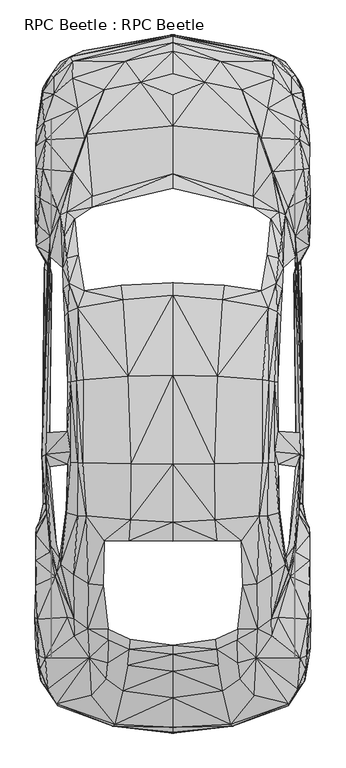
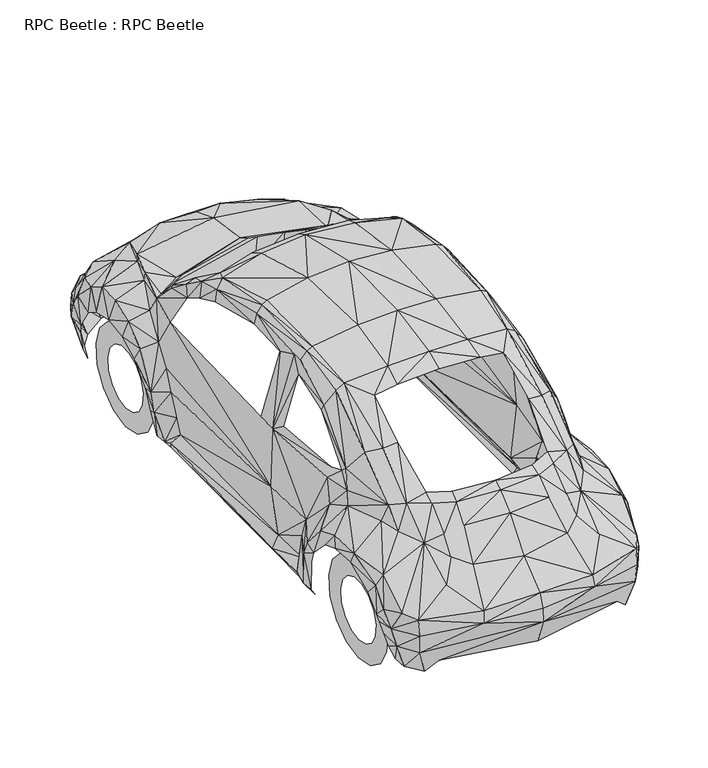
"""IFC4 building model written with IfcOpenShell, lengths in millimetres: proxy geometry, RPC Beetle : RPC Beetle."""

from ifc_helpers import new_model, si_unit, origin, place, context, project, spatial, triangles, source, transform, mapped, element, save


def rpc_beetle_rpc_beetle_3ce7ba48(model_context):
    return source(origin(), model_context, "Body", "Tessellation", [
        triangles([(0.0, -748.5640469, 521.3893959), (0.0, -720.1452873, 603.6241656), (0.0, -696.6746996, 283.1362969), (0.0, -552.698168, 738.4050739), (0.0, -753.2493713, 438.4540149), (0.0, -253.6666567, 1039.7136446), (0.0, -401.102443, 921.3971746), (0.0, -304.8115909, 1012.258271), (0.0, 339.3168975, 1395.7139351), (0.0, 448.6129515, 1442.1297066), (0.0, 778.0774343, 1504.0465668), (0.0, 1285.0166222, 1509.4764679), (0.0, 1741.0736687, 1402.3260315), (0.0, 2430.9610645, 967.1999022), (0.0, 3130.000518, 632.0428888), (0.0, 3001.4374352, 771.5091579), (0.0, 2704.2451103, 928.7536297), (0.0, 3164.1993027, 220.1684652), (0.0, 2883.1647125, 858.7358105), (0.0, 3222.5253937, 395.8040382), (0.0, 3178.9995621, 555.7633515), (0.0, 3213.942778, 530.2784609), (-338.1784132, -715.5037102, 523.0095732), (-331.0408765, -702.1482754, 593.465229), (-244.7338081, -218.0228295, 1034.0649342), (-248.9812778, -275.9549947, 1002.9312967), (-257.7389736, -368.17353, 911.8512457), (-249.0688632, 342.8199903, 1381.001025), (-285.238149, -511.5369813, 760.4306917), (-240.1360146, 460.0855433, 1426.5848705), (-236.4577871, 780.8799522, 1493.4060825), (-652.4920767, -590.2248745, 370.4943186), (-540.0870918, -593.333878, 283.4428189), (-181.240518, 2954.2772324, 806.3210592), (-253.1849819, 1278.5798058, 1496.1646351), (-379.8650402, -444.3654636, 798.2639202), (-370.9321916, -353.3292326, 889.1688366), (-367.998359, -222.2265155, 1003.4567734), (-368.3924483, -160.7037083, 1036.6922447), (-390.1553278, 342.863774, 1359.0192272), (-282.5670547, 1713.2679531, 1399.3045589), (-397.3366482, 87.4893818, 1215.3492176), (-463.1069432, -537.7663033, 704.8193333), (-271.4885704, 3072.331073, 662.6947969), (-475.7618031, -323.0713775, 849.8467455), (-463.7199872, 3085.9052444, 214.2570165), (-482.2425121, 95.7654028, 1203.3949327), (-485.0449574, -159.3024857, 1005.0769506), (-568.7247334, 3071.4988564, 546.7429356), (-493.539933, 483.2496454, 1391.2912399), (-583.2625088, 3099.3922119, 522.0462235), (-510.267146, 3132.2774139, 369.3995816), (-391.8630724, 2911.6272194, 782.7628315), (-656.3454752, -597.8440679, 480.0968582), (-660.2426937, -584.8389024, 576.2563594), (-562.2878443, -200.0695467, 879.7105476), (-560.054623, -101.457906, 987.1674334), (-512.4565473, 786.1783207, 1448.435281), (-541.7948364, 484.782219, 1359.8511532), (-563.9955889, 148.5743069, 1172.3051153), (-608.4846974, -561.2369273, 218.4607206), (-511.2742793, 1258.5246346, 1456.1858253), (-542.4078804, 784.6895308, 1430.657151), (-458.8594554, 2304.0621243, 949.0276829), (-601.0406387, -92.7439938, 893.1973698), (-503.7426533, 1765.2887604, 1320.9670441), (-546.0423243, 1253.0072388, 1441.5166626), (-603.0111217, 501.1591264, 1278.5798058), (-580.1535416, 788.8931986, 1378.7239838), (-607.2148258, 519.8568223, 1235.1416142), (-601.2595934, 965.2732029, 1337.0374294), (-712.4823103, -503.0858256, 590.4876128), (-542.6706187, 1670.0487888, 1361.1648811), (-490.6061005, 2657.8729408, 893.5038918), (-599.6394161, 778.0774343, 1307.3049419), (-598.0630225, 1243.7240845, 1343.7807678), (-639.5744785, 208.1266312, 1062.483621), (-680.4291796, -470.2006599, 218.6796571), (-538.4669146, 1966.7157097, 1180.5811363), (-580.9855039, 1248.2342743, 1401.7567348), (-644.5225777, 243.2887836, 1028.2848364), (-502.3414307, 2635.8036484, 866.0046982), (-660.7243504, 162.2363182, 955.2456173), (-690.2377378, -396.5922532, 226.824309), (-559.1350571, 2175.0175301, 1011.1634977), (-670.1826393, 140.8675371, 872.7043619), (-662.4758423, 324.2974654, 1009.4557531), (-615.0967575, 1623.4577374, 1262.1152584), (-594.6475333, 1646.0964718, 1321.2735661), (-589.4366959, 1809.6026253, 1269.4280388), (-728.8153976, -481.9797738, 373.2091965), (-751.5854467, -454.4368329, 476.550018), (-694.047389, 315.3208331, 957.7853605), (-726.5821764, -327.3188653, 735.5588814), (-622.9348692, 1777.2429726, 1192.7981232), (-564.6524165, 2445.7178673, 934.1395655), (-731.7930502, -393.877339, 324.1222944), (-571.0017383, 2444.2728973, 884.1769175), (-698.6451462, 279.8521587, 807.6347145), (-604.2809933, 1949.7695057, 1170.4659834), (-587.4224293, 3013.0852707, 200.1133485), (-690.9384218, 574.2420928, 283.6179717), (-750.2279715, -381.0035608, 396.9863425), (-627.532699, 1896.2599812, 1124.7070759), (-602.4856813, 2215.5656364, 949.1590702), (-619.4318127, 2072.8151928, 1075.2698318), (-710.4680437, 549.6329844, 448.6129515), (-764.7219995, -360.335382, 467.5295657), (-699.5209648, 762.620093, 1015.4985529), (-763.3207769, -313.2189629, 670.9270706), (-757.8472012, -390.9435428, 564.6524165), (-717.4742294, 496.2985946, 583.5690308), (-722.7288506, 461.2240276, 180.9777796), (-717.6493641, 554.4496963, 179.8830608), (-771.4654106, -341.8128571, 511.011541), (-573.9355708, 2975.4707062, 682.6185808), (-730.7859169, 375.8802907, 185.1814656), (-541.1817924, 2805.3964943, 782.9379662), (-639.7496859, 2198.4442978, 944.2547184), (-738.9305506, 551.5596474, 222.4016865), (-781.5805635, -268.7736743, 609.2290924), (-772.2974092, -106.0556904, 755.9205019), (-721.7217173, 957.7416132, 967.0247675), (-703.3305433, 810.1306377, 292.3318839), (-724.8306845, 835.0462681, 964.3536369), (-757.7596338, 370.5381022, 225.46687), (-785.3463221, -89.9415304, 695.492359), (-779.6538643, 80.9211054, 675.5686478), (-779.3910896, 89.5036484, 754.6505939), (-760.3869444, 444.1027253, 223.1460814), (-778.0774343, 192.1000477, 630.9043682), (-658.6225164, 2237.1532722, 849.7591782), (-770.939934, 345.4910846, 426.1932444), (-774.1802885, 315.1456621, 501.684603), (-781.1864742, 232.2540829, 695.886521), (-719.2257214, 810.0868177, 185.8382933), (-689.8874685, 1858.8647346, 293.9082593), (-696.6746996, 1958.8775253, 956.4279579), (-779.7414316, 377.369117, 532.3802948), (-778.1212543, 416.9976574, 439.7238865), (-745.498827, 819.5889267, 613.6517149), (-677.7143017, 2884.8285645, 670.6205486), (-697.5504456, 2077.4130226, 756.8838152), (-639.6182985, 3069.1780678, 391.6879377), (-713.0077869, 1918.2417789, 536.7153863), (-718.1748407, 1909.8781906, 192.97583), (-705.1696753, 1981.9540237, 648.2884089), (-730.7859169, 1891.093, 233.3488017), (-673.9922178, 2907.8614609, 198.6683241), (-726.8886984, 2038.9229301, 189.9544119), (-721.6340773, 1973.3715534, 189.9544119), (-678.1959583, 2982.5644592, 540.5249648), (-699.6085321, 2815.6865639, 206.1999501), (-696.3681776, 2991.5851295, 517.4046464), (-723.6484165, 2624.6813622, 787.5795433), (-699.0830555, 1882.466637, 390.3742825), (-764.8971342, 2042.1632847, 362.5686032), (-741.7768158, 2457.6720795, 808.6855951), (-716.1605742, 2965.1367439, 449.5325174), (-766.4297441, 2001.1333763, 376.580902), (-731.5740955, 2724.4313782, 727.6331297), (-771.1588886, 2084.5942703, 482.2425121), (-759.1170364, 2291.4072281, 780.0917009), (-769.0132347, 2143.3146687, 699.0392355), (-777.5520304, 2022.8525448, 494.8098046), (-742.4774271, 2846.8640213, 601.8726374), (-782.1059675, 2185.6580143, 616.4541601), (-739.5435946, 2918.4145958, 427.3755486), (-741.1199518, 2896.5202927, 519.8130023), (-750.4031061, 2804.433181, 398.0810431), (-782.2373549, 2313.1701439, 680.7357016), (-778.0774343, 2462.7953133, 693.5219124), (-759.9052151, 2786.611013, 455.2250115), (-774.1802885, 2682.8324638, 602.660816), (-780.3544756, 2589.4317696, 666.3292408), (-742.6088144, 809.1235044, 220.3874017), (0.0, 2349.0766731, 1011.1634977), (-458.8594554, 2239.9557175, 1006.6095606), (0.0, 1812.0110538, 1368.2147415), (-293.952043, 1795.8092812, 1359.1506145), (-580.2411089, 849.7154308, 1381.7892036), (338.1784132, -715.5037102, 523.0095732), (331.0408765, -702.1482754, 593.465229), (244.7338081, -218.0228295, 1034.0649342), (248.9812778, -275.9549947, 1002.9312967), (257.7389736, -368.17353, 911.8512457), (249.0688632, 342.8199903, 1381.001025), (285.238149, -511.5369813, 760.4306917), (240.1360146, 460.0855433, 1426.5848705), (236.4577871, 780.8799522, 1493.4060825), (652.4920767, -590.2248745, 370.4943186), (540.0870918, -593.333878, 283.4428189), (181.240518, 2954.2772324, 806.3210592), (253.1849819, 1278.5798058, 1496.1646351), (379.8650402, -444.3654636, 798.2639202), (370.9321916, -353.3292326, 889.1688366), (367.998359, -222.2265155, 1003.4567734), (368.3924483, -160.7037083, 1036.6922447), (390.1553278, 342.863774, 1359.0192272), (282.5670547, 1713.2679531, 1399.3045589), (397.3366482, 87.4893818, 1215.3492176), (463.1069432, -537.7663033, 704.8193333), (271.4885704, 3072.331073, 662.6947969), (475.7618031, -323.0713775, 849.8467455), (463.7199872, 3085.9052444, 214.2570165), (482.2425121, 95.7654028, 1203.3949327), (485.0449574, -159.3024857, 1005.0769506), (568.7247334, 3071.4988564, 546.7429356), (493.539933, 483.2496454, 1391.2912399), (583.2625088, 3099.3922119, 522.0462235), (510.267146, 3132.2774139, 369.3995816), (391.8630724, 2911.6272194, 782.7628315), (656.3454752, -597.8440679, 480.0968582), (660.2426937, -584.8389024, 576.2563594), (562.2878443, -200.0695467, 879.7105476), (560.054623, -101.457906, 987.1674334), (512.4565473, 786.1783207, 1448.435281), (541.7948364, 484.782219, 1359.8511532), (563.9955889, 148.5743069, 1172.3051153), (608.4846974, -561.2369273, 218.4607206), (511.2742793, 1258.5246346, 1456.1858253), (542.4078804, 784.6895308, 1430.657151), (458.8594554, 2304.0621243, 949.0276829), (601.0406387, -92.7439938, 893.1973698), (503.7426533, 1765.2887604, 1320.9670441), (546.0423243, 1253.0072388, 1441.5166626), (603.0111217, 501.1591264, 1278.5798058), (580.1535416, 788.8931986, 1378.7239838), (607.2148258, 519.8568223, 1235.1416142), (601.2595934, 965.2732029, 1337.0374294), (712.4823103, -503.0858256, 590.4876128), (542.6706187, 1670.0487888, 1361.1648811), (490.6061005, 2657.8729408, 893.5038918), (599.6394161, 778.0774343, 1307.3049419), (598.0630225, 1243.7240845, 1343.7807678), (639.5744785, 208.1266312, 1062.483621), (680.4729269, -470.2006599, 218.6796571), (538.4669146, 1966.7157097, 1180.5811363), (580.9855039, 1248.2342743, 1401.7567348), (644.5225777, 243.2887836, 1028.2848364), (502.3414307, 2635.8036484, 866.0046982), (660.7243504, 162.2363182, 955.2456173), (690.2377378, -396.5922532, 226.824309), (559.1350571, 2175.0175301, 1011.1634977), (670.1826393, 140.8675371, 872.7043619), (662.4758423, 324.2974654, 1009.4557531), (615.0967575, 1623.4577374, 1262.1152584), (594.6475333, 1646.0964718, 1321.2735661), (589.4366959, 1809.6026253, 1269.4280388), (728.8153976, -481.9797738, 373.2091965), (751.5854467, -454.4368329, 476.550018), (694.047389, 315.3208331, 957.7853605), (726.5821764, -327.3188653, 735.5588814), (622.9348692, 1777.2429726, 1192.7981232), (564.6524165, 2445.7178673, 934.1395655), (731.7930502, -393.877339, 324.1222944), (571.0017383, 2444.2728973, 884.1769175), (698.6451462, 279.8521587, 807.6347145), (604.2809933, 1949.7695057, 1170.4659834), (587.4224293, 3013.0852707, 200.1133485), (690.9384218, 574.2420928, 283.6179717), (750.2279715, -381.0035608, 396.9863425), (627.532699, 1896.2599812, 1124.7070759), (602.4856813, 2215.5656364, 949.1590702), (619.4318127, 2072.8151928, 1075.2698318), (710.4680437, 549.6329844, 448.6129515), (764.7219995, -360.335382, 467.5295657), (699.5209648, 762.620093, 1015.4985529), (763.3207769, -313.2189629, 670.9270706), (757.8472012, -390.9435428, 564.6524165), (717.4742294, 496.2985946, 583.5690308), (722.7288506, 461.2240276, 180.9777796), (717.6493641, 554.4496963, 179.8830608), (771.4654106, -341.8128571, 511.011541), (573.9355708, 2975.4707062, 682.6185808), (730.7859169, 375.8802907, 185.1814656), (541.1817924, 2805.3964943, 782.9379662), (639.7496859, 2198.4442978, 944.2547184), (738.9305506, 551.5596474, 222.4016865), (781.5805635, -268.7736743, 609.2290924), (772.2974092, -106.0556904, 755.9205019), (721.7654646, 957.7416132, 967.0247675), (703.3305433, 810.1306377, 292.3318839), (724.8306845, 835.0462681, 964.3536369), (757.7596338, 370.5381022, 225.46687), (785.3463221, -89.9415304, 695.492359), (779.6538643, 80.9211054, 675.5686478), (779.4349096, 89.5036484, 754.6505939), (760.3869444, 444.1027253, 223.1460814), (778.0774343, 192.1000477, 630.9043682), (658.6225164, 2237.1532722, 849.7591782), (770.939934, 345.4910846, 426.1932444), (774.1802885, 315.1456621, 501.684603), (781.1864742, 232.2540829, 695.886521), (719.2257214, 810.0868177, 185.8382933), (689.8874685, 1858.8647346, 293.9082593), (696.6746996, 1958.8775253, 956.4279579), (779.7414316, 377.369117, 532.3802948), (778.1212543, 416.9976574, 439.7238865), (745.498827, 819.5889267, 613.6517149), (677.7143017, 2884.8285645, 670.6205486), (697.5504456, 2077.4130226, 756.8838152), (639.6182985, 3069.1780678, 391.6879377), (713.0077869, 1918.2417789, 536.7153863), (718.1748407, 1909.8781906, 192.97583), (705.1696753, 1981.9540237, 648.2884089), (730.7859169, 1891.093, 233.3488017), (673.9922178, 2907.8614609, 198.6683241), (726.8886984, 2038.9229301, 189.9544119), (721.6340773, 1973.3715534, 189.9544119), (678.1959583, 2982.5644592, 540.5249648), (699.6085321, 2815.6865639, 206.1999501), (696.3681776, 2991.5851295, 517.4046464), (723.6484165, 2624.6813622, 787.5795433), (699.0830555, 1882.466637, 390.3742825), (764.8971342, 2042.1632847, 362.5686032), (741.7768158, 2457.6720795, 808.6855951), (716.1605742, 2965.1367439, 449.5325174), (766.4297441, 2001.1333763, 376.580902), (731.5740955, 2724.4313782, 727.6331297), (771.202636, 2084.5942703, 482.2425121), (759.1170364, 2291.4072281, 780.0917009), (769.0132347, 2143.3146687, 699.0392355), (777.5520304, 2022.8525448, 494.8098046), (742.4774271, 2846.8640213, 601.8726374), (782.1059675, 2185.6580143, 616.4541601), (739.5435946, 2918.4145958, 427.3755486), (741.1199518, 2896.5202927, 519.8130023), (750.4031061, 2804.433181, 398.0810431), (782.2373549, 2313.1701439, 680.7357016), (778.0774343, 2462.7953133, 693.5219124), (759.9052151, 2786.611013, 455.2250115), (774.1802885, 2682.8324638, 602.660816), (780.3544756, 2589.4317696, 666.3292408), (742.6088144, 809.1235044, 220.3874017), (458.8594554, 2239.9557175, 1006.6095606), (293.952043, 1795.8092812, 1359.1506145), (580.2411089, 849.7154308, 1381.7892036), (-693.1715704, 2430.2605259, 0.0015107), (-693.1715704, 2430.2605259, 117.836303), (-693.1715704, 2557.1157188, 26.9752135), (-693.1715704, 2507.7661148, 134.3007686), (-693.1715704, 2661.9892593, 103.1671675), (-693.1715704, 2571.9162689, 180.8917202), (-693.1715704, 2726.8399521, 215.4846123), (-693.1715704, 2611.544664, 249.552046), (-693.1715704, 2740.4144142, 344.4416937), (-693.1715704, 2619.820903, 328.3713083), (-693.1715704, 2700.3479645, 467.7938301), (-693.1715704, 2595.3430367, 403.7312797), (-693.1715704, 2613.5590759, 564.1284659), (-693.1715704, 2542.3151688, 462.6267763), (-693.1715704, 2495.111364, 616.8935955), (-693.1715704, 2469.8890663, 494.898898), (-693.1715704, 2365.4098331, 616.8935955), (-693.1715704, 2390.6319855, 494.898898), (-693.1715704, 2246.9619759, 564.1284659), (-693.1715704, 2318.2057377, 462.6267763), (-693.1715704, 2160.1732327, 467.7938301), (-693.1715704, 2265.1780151, 403.7312797), (-693.1715704, 2120.1067829, 344.4416937), (-693.1715704, 2240.7001488, 328.3713083), (-693.1715704, 2133.6810997, 215.4846123), (-693.1715704, 2248.9762424, 249.552046), (-693.1715704, 2198.5319378, 103.1671675), (-693.1715704, 2288.6047829, 180.8917202), (-693.1715704, 2303.4053329, 26.9752135), (-693.1715704, 2352.754937, 134.3007686), (693.1715704, 2430.2605259, 0.0015107), (693.1715704, 2430.2605259, 117.836303), (693.1715704, 2303.4053329, 26.9752135), (693.1715704, 2352.754937, 134.3007686), (693.1715704, 2198.5319378, 103.1671675), (693.1715704, 2288.6047829, 180.8917202), (693.1715704, 2133.6810997, 215.4846123), (693.1715704, 2248.9762424, 249.552046), (693.1715704, 2120.1067829, 344.4416937), (693.1715704, 2240.7001488, 328.3713083), (693.1715704, 2160.1732327, 467.7938301), (693.1715704, 2265.1780151, 403.7312797), (693.1715704, 2246.9619759, 564.1284659), (693.1715704, 2318.2057377, 462.6267763), (693.1715704, 2365.4098331, 616.8935955), (693.1715704, 2390.6319855, 494.898898), (693.1715704, 2495.111364, 616.8935955), (693.1715704, 2469.8890663, 494.898898), (693.1715704, 2613.5590759, 564.1284659), (693.1715704, 2542.3151688, 462.6267763), (693.1715704, 2700.3479645, 467.7938301), (693.1715704, 2595.3430367, 403.7312797), (693.1715704, 2740.4144142, 344.4416937), (693.1715704, 2619.820903, 328.3713083), (693.1715704, 2726.8399521, 215.4846123), (693.1715704, 2611.544664, 249.552046), (693.1715704, 2661.9892593, 103.1671675), (693.1715704, 2571.9162689, 180.8917202), (693.1715704, 2557.1157188, 26.9752135), (693.1715704, 2507.7661148, 134.3007686), (-693.1715704, -13.5744281, 0.0015107), (-693.1715704, -13.5744281, 117.836303), (-693.1715704, 113.2807944, 26.9752135), (-693.1715704, 63.9311767, 134.3007686), (-693.1715704, 218.1541986, 103.1671675), (-693.1715704, 128.0812991, 180.8917202), (-693.1715704, 283.0049277, 215.4846123), (-693.1715704, 167.7098758, 249.552046), (-693.1715704, 296.5793535, 344.4416937), (-693.1715704, 175.9858968, 328.3713083), (-693.1715704, 256.5129038, 467.7938301), (-693.1715704, 151.5081304, 403.7312797), (-693.1715704, 169.7241424, 564.1284659), (-693.1715704, 98.4802897, 462.6267763), (-693.1715704, 51.2763078, 616.8935955), (-693.1715704, 26.0541442, 494.898898), (-693.1715704, -78.425164, 616.8935955), (-693.1715704, -53.2030025, 494.898898), (-693.1715704, -196.872994, 564.1284659), (-693.1715704, -125.6291413, 462.6267763), (-693.1715704, -283.6617554, 467.7938301), (-693.1715704, -178.6569911, 403.7312797), (-693.1715704, -323.7282051, 344.4416937), (-693.1715704, -203.1347484, 328.3713083), (-693.1715704, -310.1537793, 215.4846123), (-693.1715704, -194.8587274, 249.552046), (-693.1715704, -245.3030502, 103.1671675), (-693.1715704, -155.2301507, 180.8917202), (-693.1715704, -140.429646, 26.9752135), (-693.1715704, -91.0800329, 134.3007686), (693.1715704, -13.5744281, 0.0015107), (693.1715704, -13.5744281, 117.836303), (693.1715704, -140.429646, 26.9752135), (693.1715704, -91.0800329, 134.3007686), (693.1715704, -245.3030502, 103.1671675), (693.1715704, -155.2301507, 180.8917202), (693.1715704, -310.1537793, 215.4846123), (693.1715704, -194.8587274, 249.552046), (693.1715704, -323.7282051, 344.4416937), (693.1715704, -203.1347484, 328.3713083), (693.1715704, -283.6617554, 467.7938301), (693.1715704, -178.6569911, 403.7312797), (693.1715704, -196.872994, 564.1284659), (693.1715704, -125.6291413, 462.6267763), (693.1715704, -78.425164, 616.8935955), (693.1715704, -53.2030025, 494.898898), (693.1715704, 51.2763078, 616.8935955), (693.1715704, 26.0541442, 494.898898), (693.1715704, 169.7241424, 564.1284659), (693.1715704, 98.4802897, 462.6267763), (693.1715704, 256.5129038, 467.7938301), (693.1715704, 151.5081304, 403.7312797), (693.1715704, 296.5793535, 344.4416937), (693.1715704, 175.9858968, 328.3713083), (693.1715704, 283.0049277, 215.4846123), (693.1715704, 167.7098758, 249.552046), (693.1715704, 218.1541986, 103.1671675), (693.1715704, 128.0812991, 180.8917202), (693.1715704, 113.2807944, 26.9752135), (693.1715704, 63.9311767, 134.3007686)], [[67, 58, 62], [67, 63, 58], [53, 82, 74], [34, 17, 19], [118, 82, 53], [155, 98, 82], [155, 158, 98], [34, 74, 17], [172, 155, 175], [172, 158, 155], [159, 168, 169], [166, 142, 169], [175, 161, 174], [175, 155, 161], [142, 152, 169], [154, 169, 152], [160, 145, 165], [160, 156, 145], [162, 160, 165], [162, 157, 160], [34, 53, 74], [74, 96, 64], [82, 96, 74], [82, 98, 96], [36, 29, 27], [29, 43, 24], [23, 55, 54], [23, 24, 55], [23, 2, 24], [23, 1, 2], [5, 1, 23], [134, 140, 133], [134, 139, 140], [117, 130, 113], [117, 126, 130], [113, 120, 114], [113, 130, 120], [140, 112, 107], [140, 139, 112], [92, 108, 103], [91, 103, 97], [91, 92, 103], [61, 33, 32], [84, 78, 91], [84, 91, 97], [38, 26, 25], [77, 81, 83], [63, 50, 58], [63, 59, 50], [68, 63, 69], [68, 59, 63], [181, 75, 69], [74, 64, 17], [64, 14, 17], [64, 178, 14], [178, 177, 14], [34, 19, 16], [53, 34, 44], [21, 44, 15], [21, 49, 44], [44, 34, 15], [34, 16, 15], [22, 49, 21], [22, 51, 49], [20, 51, 22], [20, 52, 51], [18, 52, 20], [18, 46, 52], [51, 152, 49], [51, 154, 152], [101, 144, 46], [144, 52, 46], [101, 159, 144], [159, 169, 154], [101, 168, 159], [101, 149, 168], [149, 170, 168], [149, 153, 170], [168, 173, 169], [168, 170, 173], [49, 142, 116], [49, 152, 142], [49, 116, 44], [116, 142, 118], [161, 155, 118], [155, 82, 118], [142, 161, 118], [158, 132, 98], [158, 163, 132], [172, 163, 158], [172, 171, 163], [98, 119, 96], [98, 132, 119], [171, 164, 163], [171, 167, 164], [163, 143, 132], [163, 164, 143], [96, 105, 64], [96, 119, 105], [105, 178, 64], [105, 85, 178], [167, 165, 164], [167, 162, 165], [165, 143, 164], [165, 147, 143], [150, 160, 157], [150, 151, 160], [151, 156, 160], [151, 148, 137], [13, 35, 12], [13, 41, 35], [12, 31, 11], [12, 35, 31], [35, 58, 31], [35, 62, 58], [11, 30, 10], [11, 31, 30], [31, 50, 30], [31, 58, 50], [10, 28, 9], [10, 30, 28], [30, 40, 28], [30, 50, 40], [125, 75, 181], [125, 109, 75], [125, 87, 109], [125, 93, 87], [123, 141, 125], [137, 141, 156], [137, 124, 141], [148, 124, 137], [148, 176, 124], [146, 176, 148], [146, 136, 176], [141, 112, 125], [112, 93, 125], [112, 99, 93], [124, 112, 141], [124, 107, 112], [124, 102, 107], [176, 102, 124], [176, 120, 102], [136, 120, 176], [136, 114, 120], [47, 40, 50], [47, 42, 40], [48, 42, 47], [48, 39, 42], [57, 47, 60], [57, 48, 47], [60, 50, 59], [60, 47, 50], [59, 77, 60], [59, 68, 77], [77, 57, 60], [77, 83, 57], [70, 77, 68], [70, 81, 77], [75, 68, 69], [75, 70, 68], [26, 6, 25], [26, 8, 6], [27, 8, 26], [27, 7, 8], [29, 7, 27], [29, 4, 7], [24, 4, 29], [24, 2, 4], [32, 5, 23], [33, 5, 32], [33, 3, 5], [32, 23, 54], [55, 45, 72], [55, 24, 43], [99, 83, 93], [99, 86, 83], [135, 86, 99], [135, 129, 86], [131, 129, 135], [131, 128, 129], [93, 81, 87], [93, 83, 81], [128, 122, 129], [128, 127, 122], [122, 86, 129], [122, 65, 86], [86, 57, 83], [86, 65, 57], [127, 110, 122], [127, 121, 110], [110, 94, 122], [122, 94, 65], [94, 56, 65], [56, 57, 65], [56, 48, 57], [56, 45, 48], [94, 45, 56], [115, 110, 121], [115, 111, 110], [111, 94, 110], [111, 72, 94], [108, 92, 115], [92, 111, 115], [78, 32, 91], [78, 61, 32], [45, 38, 48], [45, 37, 38], [37, 26, 38], [37, 27, 26], [36, 27, 37], [134, 135, 139], [134, 131, 135], [139, 99, 112], [139, 135, 99], [126, 140, 130], [126, 133, 140], [130, 107, 120], [130, 140, 107], [120, 107, 102], [45, 36, 37], [92, 55, 72], [92, 54, 55], [91, 54, 92], [91, 32, 54], [92, 72, 111], [72, 45, 94], [43, 45, 55], [43, 36, 45], [43, 29, 36], [79, 90, 66], [79, 100, 90], [90, 73, 66], [85, 100, 79], [85, 106, 100], [85, 105, 106], [105, 119, 106], [95, 88, 89], [90, 89, 73], [89, 67, 73], [73, 67, 62], [89, 76, 80], [89, 80, 67], [88, 76, 89], [73, 35, 41], [73, 62, 35], [69, 63, 181], [80, 63, 67], [76, 71, 80], [146, 148, 151], [141, 147, 145], [151, 137, 156], [173, 166, 169], [173, 174, 166], [166, 174, 161], [166, 161, 142], [52, 144, 51], [144, 154, 51], [144, 159, 154], [116, 53, 44], [116, 118, 53], [119, 143, 138], [143, 119, 132], [143, 147, 138], [138, 104, 119], [119, 104, 106], [104, 100, 106], [104, 90, 100], [104, 95, 90], [95, 89, 90], [25, 39, 38], [38, 39, 48], [141, 138, 147], [156, 141, 145], [165, 145, 147], [41, 179, 180], [41, 13, 179], [66, 41, 180], [66, 73, 41], [123, 125, 71], [125, 181, 71], [71, 181, 80], [181, 63, 80], [138, 141, 123], [226, 221, 217], [226, 217, 222], [212, 233, 241], [193, 19, 17], [277, 212, 241], [314, 241, 257], [314, 257, 317], [193, 17, 233], [331, 334, 314], [331, 314, 317], [318, 328, 327], [325, 328, 301], [334, 333, 320], [334, 320, 314], [301, 328, 311], [313, 311, 328], [319, 324, 304], [319, 304, 315], [321, 324, 319], [321, 319, 316], [193, 233, 212], [233, 223, 255], [241, 233, 255], [241, 255, 257], [195, 186, 188], [188, 183, 202], [182, 213, 214], [182, 214, 183], [182, 183, 2], [182, 2, 1], [5, 182, 1], [293, 292, 299], [293, 299, 298], [276, 272, 289], [276, 289, 285], [272, 273, 279], [272, 279, 289], [299, 266, 271], [299, 271, 298], [251, 262, 267], [250, 256, 262], [250, 262, 251], [220, 191, 192], [243, 250, 237], [243, 256, 250], [197, 184, 185], [236, 242, 240], [222, 217, 209], [222, 209, 218], [227, 228, 222], [227, 222, 218], [338, 228, 234], [233, 17, 223], [223, 17, 14], [223, 14, 336], [336, 14, 177], [193, 16, 19], [212, 203, 193], [21, 15, 203], [21, 203, 208], [203, 15, 193], [193, 15, 16], [22, 21, 208], [22, 208, 210], [20, 22, 210], [20, 210, 211], [18, 20, 211], [18, 211, 205], [210, 208, 311], [210, 311, 313], [260, 205, 303], [303, 205, 211], [260, 303, 318], [318, 313, 328], [260, 318, 327], [260, 327, 308], [308, 327, 329], [308, 329, 312], [327, 328, 332], [327, 332, 329], [208, 275, 301], [208, 301, 311], [208, 203, 275], [275, 277, 301], [320, 277, 314], [314, 277, 241], [301, 277, 320], [317, 257, 291], [317, 291, 322], [331, 317, 322], [331, 322, 330], [257, 255, 278], [257, 278, 291], [330, 322, 323], [330, 323, 326], [322, 291, 302], [322, 302, 323], [255, 223, 264], [255, 264, 278], [264, 223, 336], [264, 336, 244], [326, 323, 324], [326, 324, 321], [324, 323, 302], [324, 302, 306], [309, 316, 319], [309, 319, 310], [310, 319, 315], [310, 296, 307], [13, 12, 194], [13, 194, 200], [12, 11, 190], [12, 190, 194], [194, 190, 217], [194, 217, 221], [11, 10, 189], [11, 189, 190], [190, 189, 209], [190, 209, 217], [10, 9, 187], [10, 187, 189], [189, 187, 199], [189, 199, 209], [284, 338, 234], [284, 234, 268], [284, 268, 246], [284, 246, 252], [282, 284, 300], [296, 315, 300], [296, 300, 283], [307, 296, 283], [307, 283, 335], [305, 307, 335], [305, 335, 295], [300, 284, 271], [271, 284, 252], [271, 252, 258], [283, 300, 271], [283, 271, 266], [283, 266, 261], [335, 283, 261], [335, 261, 279], [295, 335, 279], [295, 279, 273], [206, 209, 199], [206, 199, 201], [207, 206, 201], [207, 201, 198], [216, 219, 206], [216, 206, 207], [219, 218, 209], [219, 209, 206], [218, 219, 236], [218, 236, 227], [236, 219, 216], [236, 216, 242], [229, 227, 236], [229, 236, 240], [234, 228, 227], [234, 227, 229], [185, 184, 6], [185, 6, 8], [186, 185, 8], [186, 8, 7], [188, 186, 7], [188, 7, 4], [183, 188, 4], [183, 4, 2], [191, 182, 5], [192, 191, 5], [192, 5, 3], [191, 213, 182], [214, 231, 204], [214, 202, 183], [258, 252, 242], [258, 242, 245], [294, 258, 245], [294, 245, 288], [290, 294, 288], [290, 288, 287], [252, 246, 240], [252, 240, 242], [287, 288, 281], [287, 281, 286], [281, 288, 245], [281, 245, 224], [245, 242, 216], [245, 216, 224], [286, 281, 269], [286, 269, 280], [269, 281, 253], [281, 224, 253], [253, 224, 215], [215, 224, 216], [215, 216, 207], [215, 207, 204], [253, 215, 204], [274, 280, 269], [274, 269, 270], [270, 269, 253], [270, 253, 231], [267, 274, 251], [251, 274, 270], [237, 250, 191], [237, 191, 220], [204, 207, 197], [204, 197, 196], [196, 197, 185], [196, 185, 186], [195, 196, 186], [293, 298, 294], [293, 294, 290], [298, 271, 258], [298, 258, 294], [285, 289, 299], [285, 299, 292], [289, 279, 266], [289, 266, 299], [279, 261, 266], [204, 196, 195], [251, 231, 214], [251, 214, 213], [250, 251, 213], [250, 213, 191], [251, 270, 231], [231, 253, 204], [202, 214, 204], [202, 204, 195], [202, 195, 188], [238, 225, 249], [238, 249, 259], [249, 225, 232], [244, 238, 259], [244, 259, 265], [244, 265, 264], [264, 265, 278], [254, 248, 247], [249, 232, 248], [248, 232, 226], [232, 221, 226], [248, 239, 235], [248, 226, 239], [247, 248, 235], [232, 200, 194], [232, 194, 221], [228, 338, 222], [239, 226, 222], [235, 239, 230], [305, 310, 307], [300, 304, 306], [310, 315, 296], [332, 328, 325], [332, 325, 333], [325, 320, 333], [325, 301, 320], [211, 210, 303], [303, 210, 313], [303, 313, 318], [275, 203, 212], [275, 212, 277], [278, 297, 302], [302, 291, 278], [302, 297, 306], [297, 278, 263], [278, 265, 263], [263, 265, 259], [263, 259, 249], [263, 249, 254], [254, 249, 248], [184, 197, 198], [197, 207, 198], [300, 306, 297], [315, 304, 300], [324, 306, 304], [200, 337, 179], [200, 179, 13], [225, 337, 200], [225, 200, 232], [282, 230, 284], [284, 230, 338], [230, 239, 338], [338, 239, 222], [297, 282, 300], [339, 342, 341], [339, 340, 342], [341, 344, 343], [341, 342, 344], [343, 346, 345], [343, 344, 346], [345, 348, 347], [345, 346, 348], [347, 350, 349], [347, 348, 350], [349, 352, 351], [349, 350, 352], [351, 354, 353], [351, 352, 354], [353, 356, 355], [353, 354, 356], [355, 358, 357], [355, 356, 358], [357, 360, 359], [357, 358, 360], [359, 362, 361], [359, 360, 362], [361, 364, 363], [361, 362, 364], [363, 366, 365], [363, 364, 366], [365, 368, 367], [365, 366, 368], [367, 340, 339], [367, 368, 340], [369, 372, 371], [369, 370, 372], [371, 374, 373], [371, 372, 374], [373, 376, 375], [373, 374, 376], [375, 378, 377], [375, 376, 378], [377, 380, 379], [377, 378, 380], [379, 382, 381], [379, 380, 382], [381, 384, 383], [381, 382, 384], [383, 386, 385], [383, 384, 386], [385, 388, 387], [385, 386, 388], [387, 390, 389], [387, 388, 390], [389, 392, 391], [389, 390, 392], [391, 394, 393], [391, 392, 394], [393, 396, 395], [393, 394, 396], [395, 398, 397], [395, 396, 398], [397, 370, 369], [397, 398, 370], [399, 402, 401], [399, 400, 402], [401, 404, 403], [401, 402, 404], [403, 406, 405], [403, 404, 406], [405, 408, 407], [405, 406, 408], [407, 410, 409], [407, 408, 410], [409, 412, 411], [409, 410, 412], [411, 414, 413], [411, 412, 414], [413, 416, 415], [413, 414, 416], [415, 418, 417], [415, 416, 418], [417, 420, 419], [417, 418, 420], [419, 422, 421], [419, 420, 422], [421, 424, 423], [421, 422, 424], [423, 426, 425], [423, 424, 426], [425, 428, 427], [425, 426, 428], [427, 400, 399], [427, 428, 400], [429, 432, 431], [429, 430, 432], [431, 434, 433], [431, 432, 434], [433, 436, 435], [433, 434, 436], [435, 438, 437], [435, 436, 438], [437, 440, 439], [437, 438, 440], [439, 442, 441], [439, 440, 442], [441, 444, 443], [441, 442, 444], [443, 446, 445], [443, 444, 446], [445, 448, 447], [445, 446, 448], [447, 450, 449], [447, 448, 450], [449, 452, 451], [449, 450, 452], [451, 454, 453], [451, 452, 454], [453, 456, 455], [453, 454, 456], [455, 458, 457], [455, 456, 458], [457, 430, 429], [457, 458, 430]], closed=False),
    ])


if __name__ == "__main__":
    model = new_model("IFC4")
    model_context = context("Model", 3, world=origin())
    ifc_project = project(units=[si_unit("LENGTHUNIT", "METRE", prefix="MILLI")], contexts=[model_context])
    site = spatial("IfcSite", under=ifc_project)
    building = spatial("IfcBuilding", under=site)
    placement = place(None, origin())
    rpc_beetle_rpc_beetle_shape = rpc_beetle_rpc_beetle_3ce7ba48(model_context)
    element("IfcBuildingElementProxy", 1, Name="RPC Beetle : RPC Beetle", ObjectType="RPC Beetle : RPC Beetle", at=placement, inside=building, context=model_context, shape_type="MappedRepresentation", body=[
        mapped(rpc_beetle_rpc_beetle_shape, transform((0.0, 0.0, 0.0), x_axis=(1.0, 0.0, 0.0), y_axis=(0.0, 1.0, 0.0), z_axis=(0.0, 0.0, 1.0))),
    ])
    save(model, "model.ifc")

# Revit data of these elements
# Type "RPC Beetle : RPC Beetle"
#   built-in parameter 1005195 = "RPC-16-0U6E-L4EG-ENH1-J3KF-SVEL-0TX4-C0"
#   Height = 0
